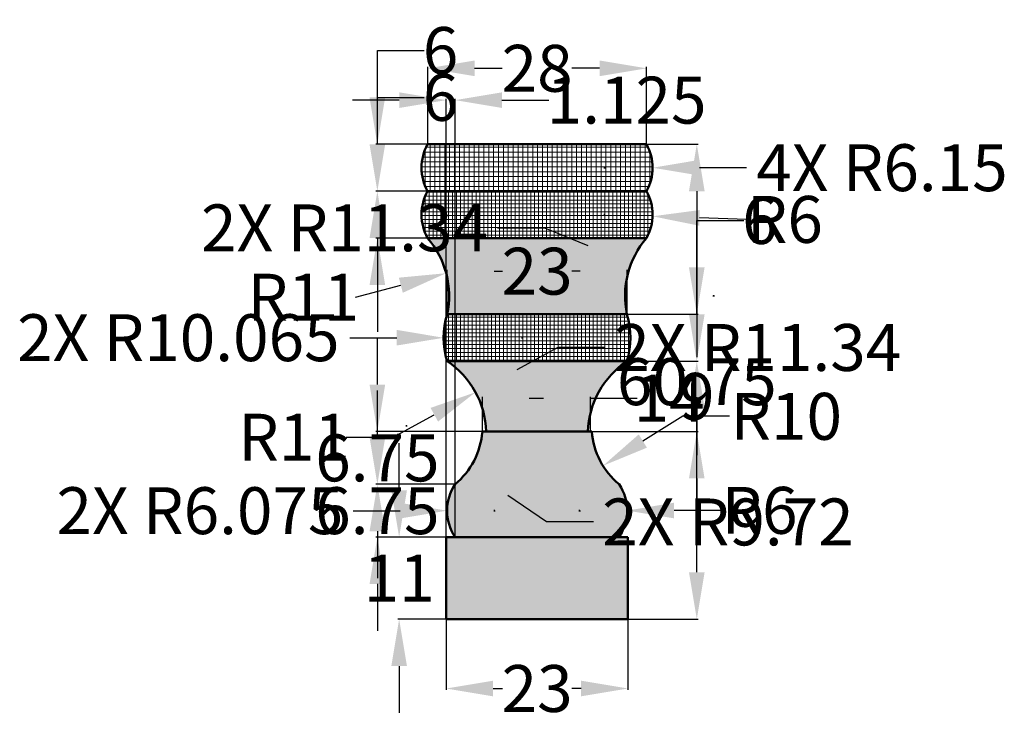
# Model space of a CAD drawing. Units: millimetres. Extents: x 141 to 267, y 101 to 190.
import ezdxf

# ---------------------------------------------------------------- set-up
doc = ezdxf.new("R2010")
doc.units = ezdxf.units.MM
doc.header["$MEASUREMENT"] = 0
for name, color, linetype, lineweight in [('M-DIMS', 2, 'Continuous', 25), ('M-HATC', 8, 'Continuous', 18), ('M-OUTL', 7, 'Continuous', 50)]:
    doc.layers.add(name, color=color, linetype=linetype, lineweight=lineweight)
doc.styles.get("Standard").update_dxf_attribs({"font": 'arial.ttf'})
doc.dimstyles.get("Standard").update_dxf_attribs({"dimtxt": 6, "dimasz": 6, "dimexe": 0.18, "dimexo": 0.0625, "dimgap": 0.09, "dimtad": 0, "dimtih": 1, "dimtoh": 1, "dimdec": 0, "dimzin": 0, "dimdsep": 46, "dimtxsty": 'Standard', "dimcen": 0.09, "dimadec": 0, "dimazin": 0, "dimtfac": 1, "dimtdec": 0, "dimtofl": 0, "dimtmove": 0, "dimatfit": 3, "dimfxl": 1, "dimtolj": 1, "dimtzin": 0, "dimarcsym": 0})

# ---------------------------------------------------------------- blocks, each defined once
blk = doc.blocks.new('*D1')
at = {"layer": 'Defpoints', "color": 0, "transparency": 16777216}
for p in [(195.71, 157.64), (184.75, 154.74)]:
    blk.add_point(p, dxfattribs=at)
at = {"layer": 'M-DIMS', "color": 0, "lineweight": -2, "transparency": 16777216}
blk.add_line((184.11, 154.57), (189.91, 156.11), dxfattribs=at)
at = {"layer": 'M-DIMS', "color": 0, "transparency": 16777216}
blk.add_solid([(189.66, 157.07), (190.17, 155.14), (195.71, 157.64)], dxfattribs=at)
at = {"layer": 'M-DIMS', "color": 0, "transparency": 16777216, "insert": (177.43, 154.57), "char_height": 6, "attachment_point": 5}
blk.add_mtext('\\A1;R11', dxfattribs=at)
blk = doc.blocks.new('*D2')
at = {"layer": 'Defpoints', "color": 0, "transparency": 16777216}
for p in [(199.47, 142.41), (189.51, 136.98)]:
    blk.add_point(p, dxfattribs=at)
at = {"layer": 'M-DIMS', "color": 0, "lineweight": -2, "transparency": 16777216}
for p, q in [((188.93, 136.66), (194.2, 139.54)), ((182.93, 136.66), (188.93, 136.66))]:
    blk.add_line(p, q, dxfattribs=at)
at = {"layer": 'M-DIMS', "color": 0, "transparency": 16777216}
blk.add_solid([(193.72, 140.41), (194.68, 138.66), (199.47, 142.41)], dxfattribs=at)
at = {"layer": 'M-DIMS', "color": 0, "transparency": 16777216, "insert": (176.25, 136.66), "char_height": 6, "attachment_point": 5}
blk.add_mtext('\\A1;R11', dxfattribs=at)
blk = doc.blocks.new('*D3')
at = {"layer": 'Defpoints', "color": 0, "transparency": 16777216}
for p in [(224.04, 138.13), (215.78, 133.01)]:
    blk.add_point(p, dxfattribs=at)
at = {"layer": 'M-DIMS', "color": 0, "lineweight": -2, "transparency": 16777216}
for p, q in [((225.98, 139.33), (220.88, 136.17)), ((231.98, 139.33), (225.98, 139.33))]:
    blk.add_line(p, q, dxfattribs=at)
at = {"layer": 'M-DIMS', "color": 0, "transparency": 16777216}
blk.add_solid([(220.35, 137.02), (221.4, 135.32), (215.78, 133.01)], dxfattribs=at)
at = {"layer": 'M-DIMS', "color": 0, "transparency": 16777216, "insert": (239.22, 139.33), "char_height": 6, "attachment_point": 5}
blk.add_mtext('\\A1;R10', dxfattribs=at)
blk = doc.blocks.new('*D4')
at = {"layer": 'Defpoints', "color": 0, "transparency": 16777216}
for p in [(212.79, 127.26), (218.87, 127.27)]:
    blk.add_point(p, dxfattribs=at)
at = {"layer": 'M-DIMS', "color": 0, "lineweight": -2, "transparency": 16777216}
for p, q in [((212.7, 127.26), (212.88, 127.26)), ((212.79, 127.17), (212.79, 127.35)), ((230.87, 127.3), (224.87, 127.28))]:
    blk.add_line(p, q, dxfattribs=at)
at = {"layer": 'M-DIMS', "color": 0, "transparency": 16777216}
blk.add_solid([(224.87, 128.28), (224.87, 126.28), (218.87, 127.27)], dxfattribs=at)
at = {"layer": 'M-DIMS', "color": 0, "transparency": 16777216, "insert": (235.8, 127.3), "char_height": 6, "attachment_point": 5}
blk.add_mtext('\\A1;R6', dxfattribs=at)
blk = doc.blocks.new('*D5')
at = {"layer": 'Defpoints', "color": 0, "transparency": 16777216}
for p in [(215.98, 165.13), (222.12, 164.92)]:
    blk.add_point(p, dxfattribs=at)
at = {"layer": 'M-DIMS', "color": 0, "lineweight": -2, "transparency": 16777216}
for p, q in [((215.89, 165.13), (216.07, 165.13)), ((215.98, 165.04), (215.98, 165.22)), ((234.12, 164.52), (228.12, 164.72))]:
    blk.add_line(p, q, dxfattribs=at)
at = {"layer": 'M-DIMS', "color": 0, "transparency": 16777216}
blk.add_solid([(228.15, 165.72), (228.09, 163.72), (222.12, 164.92)], dxfattribs=at)
at = {"layer": 'M-DIMS', "color": 0, "transparency": 16777216, "insert": (239.04, 164.52), "char_height": 6, "attachment_point": 5}
blk.add_mtext('\\A1;R6', dxfattribs=at)
blk = doc.blocks.new('*D6')
at = {"layer": 'Defpoints', "color": 0, "transparency": 16777216}
for p in [(195.72, 113.38), (218.97, 113.38), (218.97, 104.51)]:
    blk.add_point(p, dxfattribs=at)
at = {"layer": 'M-DIMS', "color": 0, "lineweight": -2, "transparency": 16777216}
for p, q in [((195.72, 113.32), (195.72, 104.33)), ((218.97, 113.32), (218.97, 104.33)), ((201.72, 104.51), (202.91, 104.51)), ((212.97, 104.51), (211.78, 104.51))]:
    blk.add_line(p, q, dxfattribs=at)
at = {"layer": 'M-DIMS', "color": 0, "transparency": 16777216}
for points in [[(201.72, 105.51), (201.72, 103.51), (195.72, 104.51)], [(212.97, 105.51), (212.97, 103.51), (218.97, 104.51)]]:
    blk.add_solid(points, dxfattribs=at)
at = {"layer": 'M-DIMS', "color": 0, "transparency": 16777216, "insert": (207.35, 104.51), "char_height": 6, "attachment_point": 5}
blk.add_mtext('\\A1;23', dxfattribs=at)
blk = doc.blocks.new('*D7')
at = {"layer": 'Defpoints', "color": 0, "transparency": 16777216}
for p in [(218.97, 123.88), (189.7, 113.38), (218.97, 113.38)]:
    blk.add_point(p, dxfattribs=at)
at = {"layer": 'M-DIMS', "color": 0, "lineweight": -2, "transparency": 16777216}
for p, q in [((189.7, 129.88), (189.7, 135.88)), ((218.91, 123.88), (189.52, 123.88)), ((218.91, 113.38), (189.52, 113.38)), ((189.7, 107.38), (189.7, 101.38))]:
    blk.add_line(p, q, dxfattribs=at)
at = {"layer": 'M-DIMS', "color": 0, "transparency": 16777216}
for points in [[(188.7, 129.88), (190.7, 129.88), (189.7, 123.88)], [(188.7, 107.38), (190.7, 107.38), (189.7, 113.38)]]:
    blk.add_solid(points, dxfattribs=at)
at = {"layer": 'M-DIMS', "color": 0, "transparency": 16777216, "insert": (189.7, 118.63), "char_height": 6, "attachment_point": 5}
blk.add_mtext('\\A1;11', dxfattribs=at)
blk = doc.blocks.new('*D8')
at = {"layer": 'Defpoints', "color": 0, "transparency": 16777216}
for p in [(221.35, 183.85), (193.35, 174.13), (221.35, 174.13)]:
    blk.add_point(p, dxfattribs=at)
at = {"layer": 'M-DIMS', "color": 0, "lineweight": -2, "transparency": 16777216}
for p, q in [((193.35, 174.2), (193.35, 184.03)), ((221.35, 174.2), (221.35, 184.03)), ((199.35, 183.85), (202.9, 183.85)), ((215.35, 183.85), (211.79, 183.85))]:
    blk.add_line(p, q, dxfattribs=at)
at = {"layer": 'M-DIMS', "color": 0, "transparency": 16777216}
for points in [[(199.35, 184.85), (199.35, 182.85), (193.35, 183.85)], [(215.35, 184.85), (215.35, 182.85), (221.35, 183.85)]]:
    blk.add_solid(points, dxfattribs=at)
at = {"layer": 'M-DIMS', "color": 0, "transparency": 16777216, "insert": (207.35, 183.85), "char_height": 6, "attachment_point": 5}
blk.add_mtext('\\A1;28', dxfattribs=at)
blk = doc.blocks.new('*D9')
at = {"layer": 'Defpoints', "color": 0, "transparency": 16777216}
for p in [(214.16, 141.66), (200.35, 137.38), (214.16, 137.38)]:
    blk.add_point(p, dxfattribs=at)
at = {"layer": 'M-DIMS', "color": 0, "lineweight": -2, "transparency": 16777216}
for p, q in [((200.35, 137.45), (200.35, 141.84)), ((206.35, 141.66), (208.16, 141.66)), ((214.16, 137.45), (214.16, 141.84)), ((214.16, 141.66), (220.16, 141.66))]:
    blk.add_line(p, q, dxfattribs=at)
at = {"layer": 'M-DIMS', "color": 0, "transparency": 16777216}
for points in [[(206.35, 142.66), (206.35, 140.66), (200.35, 141.66)], [(208.16, 142.66), (208.16, 140.66), (214.16, 141.66)]]:
    blk.add_solid(points, dxfattribs=at)
at = {"layer": 'M-DIMS', "color": 0, "transparency": 16777216, "insert": (224.25, 141.66), "char_height": 6, "attachment_point": 5}
blk.add_mtext('\\A1;14', dxfattribs=at)
blk = doc.blocks.new('*D10')
at = {"layer": 'Defpoints', "color": 0, "transparency": 16777216}
for p in [(218.85, 157.9), (195.85, 152.38), (218.85, 152.38)]:
    blk.add_point(p, dxfattribs=at)
at = {"layer": 'M-DIMS', "color": 0, "lineweight": -2, "transparency": 16777216}
for p, q in [((195.85, 152.45), (195.85, 158.08)), ((201.85, 157.9), (202.91, 157.9)), ((212.85, 157.9), (211.78, 157.9)), ((218.85, 152.45), (218.85, 158.08))]:
    blk.add_line(p, q, dxfattribs=at)
at = {"layer": 'M-DIMS', "color": 0, "transparency": 16777216}
for points in [[(201.85, 158.9), (201.85, 156.9), (195.85, 157.9)], [(212.85, 158.9), (212.85, 156.9), (218.85, 157.9)]]:
    blk.add_solid(points, dxfattribs=at)
at = {"layer": 'M-DIMS', "color": 0, "transparency": 16777216, "insert": (207.35, 157.9), "char_height": 6, "attachment_point": 5}
blk.add_mtext('\\A1;23', dxfattribs=at)
blk = doc.blocks.new('*D11')
at = {"layer": 'Defpoints', "color": 0, "transparency": 16777216}
for p in [(221.35, 174.13), (227.78, 174.13), (218.97, 113.38)]:
    blk.add_point(p, dxfattribs=at)
at = {"layer": 'M-DIMS', "color": 0, "lineweight": -2, "transparency": 16777216}
for p, q in [((221.41, 174.13), (227.96, 174.13)), ((227.78, 168.13), (227.78, 146.91)), ((227.78, 119.38), (227.78, 140.61)), ((219.03, 113.38), (227.96, 113.38))]:
    blk.add_line(p, q, dxfattribs=at)
at = {"layer": 'M-DIMS', "color": 0, "transparency": 16777216}
for points in [[(226.78, 168.13), (228.78, 168.13), (227.78, 174.13)], [(226.78, 119.38), (228.78, 119.38), (227.78, 113.38)]]:
    blk.add_solid(points, dxfattribs=at)
at = {"layer": 'M-DIMS', "color": 0, "transparency": 16777216, "insert": (227.78, 143.76), "char_height": 6, "attachment_point": 5}
blk.add_mtext('\\A1;60.75', dxfattribs=at)
blk = doc.blocks.new('*D12')
at = {"layer": 'Defpoints', "color": 0, "transparency": 16777216}
for p in [(186.914449, 130.634532), (196.84579, 130.634532), (196.84579, 123.884532)]:
    blk.add_point(p, dxfattribs=at)
at = {"layer": 'M-DIMS', "color": 0, "lineweight": -2, "transparency": 16777216}
for p, q in [((186.914449, 136.634532), (186.914449, 142.634532)), ((196.78329, 130.634532), (186.734449, 130.634532)), ((196.78329, 123.884532), (186.734449, 123.884532)), ((186.914449, 117.884532), (186.914449, 111.884532))]:
    blk.add_line(p, q, dxfattribs=at)
at = {"layer": 'M-DIMS', "color": 0, "transparency": 16777216}
for points in [[(185.914449, 136.634532), (187.914449, 136.634532), (186.914449, 130.634532)], [(185.914449, 117.884532), (187.914449, 117.884532), (186.914449, 123.884532)]]:
    blk.add_solid(points, dxfattribs=at)
at = {"layer": 'M-DIMS', "color": 0, "transparency": 16777216, "insert": (186.914449, 127.259532), "char_height": 6, "attachment_point": 5}
blk.add_mtext('\\A1;6.75', dxfattribs=at)
blk = doc.blocks.new('*D13')
at = {"layer": 'Defpoints', "color": 0, "transparency": 16777216}
for p in [(186.914449, 137.384532), (200.34579, 137.384532), (196.84579, 130.634532)]:
    blk.add_point(p, dxfattribs=at)
at = {"layer": 'M-DIMS', "color": 0, "lineweight": -2, "transparency": 16777216}
for p, q in [((186.914449, 143.384532), (186.914449, 149.384532)), ((200.28329, 137.384532), (186.734449, 137.384532)), ((196.78329, 130.634532), (186.734449, 130.634532)), ((186.914449, 124.634532), (186.914449, 118.634532))]:
    blk.add_line(p, q, dxfattribs=at)
at = {"layer": 'M-DIMS', "color": 0, "transparency": 16777216}
for points in [[(185.914449, 143.384532), (187.914449, 143.384532), (186.914449, 137.384532)], [(185.914449, 124.634532), (187.914449, 124.634532), (186.914449, 130.634532)]]:
    blk.add_solid(points, dxfattribs=at)
at = {"layer": 'M-DIMS', "color": 0, "transparency": 16777216, "insert": (186.914449, 134.009532), "char_height": 6, "attachment_point": 5}
blk.add_mtext('\\A1;6.75', dxfattribs=at)
blk = doc.blocks.new('*D14')
at = {"layer": 'Defpoints', "color": 0, "transparency": 16777216}
for p in [(218.84579, 146.384532), (227.777131, 146.384532), (214.34579, 137.384532)]:
    blk.add_point(p, dxfattribs=at)
at = {"layer": 'M-DIMS', "color": 0, "lineweight": -2, "transparency": 16777216}
for p, q in [((227.777131, 152.384532), (227.777131, 158.384532)), ((218.90829, 146.384532), (227.957131, 146.384532)), ((214.40829, 137.384532), (227.957131, 137.384532)), ((227.777131, 131.384532), (227.777131, 125.384532))]:
    blk.add_line(p, q, dxfattribs=at)
at = {"layer": 'M-DIMS', "color": 0, "transparency": 16777216}
for points in [[(226.777131, 152.384532), (228.777131, 152.384532), (227.777131, 146.384532)], [(226.777131, 131.384532), (228.777131, 131.384532), (227.777131, 137.384532)]]:
    blk.add_solid(points, dxfattribs=at)
at = {"layer": 'M-DIMS', "color": 0, "transparency": 16777216, "insert": (227.777131, 141.884532), "char_height": 6, "attachment_point": 5}
blk.add_mtext('\\A1;9', dxfattribs=at)
blk = doc.blocks.new('*D15')
at = {"layer": 'Defpoints', "color": 0, "transparency": 16777216}
for p in [(196.85, 179.78), (195.72, 123.88), (196.85, 123.88)]:
    blk.add_point(p, dxfattribs=at)
at = {"layer": 'M-DIMS', "color": 0, "lineweight": -2, "transparency": 16777216}
for p, q in [((189.72, 179.78), (183.72, 179.78)), ((195.72, 123.95), (195.72, 179.96)), ((196.85, 123.95), (196.85, 179.96)), ((202.85, 179.78), (208.85, 179.78))]:
    blk.add_line(p, q, dxfattribs=at)
at = {"layer": 'M-DIMS', "color": 0, "transparency": 16777216}
for points in [[(189.72, 180.78), (189.72, 178.78), (195.72, 179.78)], [(202.85, 180.78), (202.85, 178.78), (196.85, 179.78)]]:
    blk.add_solid(points, dxfattribs=at)
at = {"layer": 'M-DIMS', "color": 0, "transparency": 16777216, "insert": (218.8, 179.78), "char_height": 6, "attachment_point": 5}
blk.add_mtext('\\A1;1.125', dxfattribs=at)
blk = doc.blocks.new('*D16')
at = {"layer": 'Defpoints', "color": 0, "transparency": 16777216}
for p in [(218.85, 152.38), (227.78, 152.38), (218.85, 146.38)]:
    blk.add_point(p, dxfattribs=at)
at = {"layer": 'M-DIMS', "color": 0, "lineweight": -2, "transparency": 16777216}
for p, q in [((227.78, 158.38), (227.78, 164.38)), ((227.78, 164.38), (233.78, 164.38)), ((218.91, 152.38), (227.96, 152.38)), ((218.91, 146.38), (227.96, 146.38)), ((227.78, 140.38), (227.78, 134.38))]:
    blk.add_line(p, q, dxfattribs=at)
at = {"layer": 'M-DIMS', "color": 0, "transparency": 16777216}
for points in [[(226.78, 158.38), (228.78, 158.38), (227.78, 152.38)], [(226.78, 140.38), (228.78, 140.38), (227.78, 146.38)]]:
    blk.add_solid(points, dxfattribs=at)
at = {"layer": 'M-DIMS', "color": 0, "transparency": 16777216, "insert": (235.85, 164.38), "char_height": 6, "attachment_point": 5}
blk.add_mtext('\\A1;6', dxfattribs=at)
blk = doc.blocks.new('*D17')
at = {"layer": 'Defpoints', "color": 0, "transparency": 16777216}
for p in [(186.91, 168.13), (193.35, 168.13), (193.35, 162.13)]:
    blk.add_point(p, dxfattribs=at)
at = {"layer": 'M-DIMS', "color": 0, "lineweight": -2, "transparency": 16777216}
for p, q in [((186.91, 174.13), (186.91, 180.13)), ((186.91, 180.13), (192.91, 180.13)), ((193.28, 168.13), (186.73, 168.13)), ((193.28, 162.13), (186.73, 162.13)), ((186.91, 156.13), (186.91, 150.13))]:
    blk.add_line(p, q, dxfattribs=at)
at = {"layer": 'M-DIMS', "color": 0, "transparency": 16777216}
for points in [[(185.91, 174.13), (187.91, 174.13), (186.91, 168.13)], [(185.91, 156.13), (187.91, 156.13), (186.91, 162.13)]]:
    blk.add_solid(points, dxfattribs=at)
at = {"layer": 'M-DIMS', "color": 0, "transparency": 16777216, "insert": (194.99, 180.13), "char_height": 6, "attachment_point": 5}
blk.add_mtext('\\A1;6', dxfattribs=at)
blk = doc.blocks.new('*D18')
at = {"layer": 'Defpoints', "color": 0, "transparency": 16777216}
for p in [(186.91, 174.13), (193.35, 174.13), (193.35, 168.13)]:
    blk.add_point(p, dxfattribs=at)
at = {"layer": 'M-DIMS', "color": 0, "lineweight": -2, "transparency": 16777216}
for p, q in [((186.91, 180.13), (186.91, 186.13)), ((186.91, 186.13), (192.91, 186.13)), ((193.28, 174.13), (186.73, 174.13)), ((193.28, 168.13), (186.73, 168.13)), ((186.91, 162.13), (186.91, 156.13))]:
    blk.add_line(p, q, dxfattribs=at)
at = {"layer": 'M-DIMS', "color": 0, "transparency": 16777216}
for points in [[(185.91, 180.13), (187.91, 180.13), (186.91, 174.13)], [(185.91, 162.13), (187.91, 162.13), (186.91, 168.13)]]:
    blk.add_solid(points, dxfattribs=at)
at = {"layer": 'M-DIMS', "color": 0, "transparency": 16777216, "insert": (194.99, 186.13), "char_height": 6, "attachment_point": 5}
blk.add_mtext('\\A1;6', dxfattribs=at)
blk = doc.blocks.new('*D19')
at = {"layer": 'Defpoints', "color": 0, "transparency": 16777216}
for p in [(195.39, 149.38), (205.45, 149.38)]:
    blk.add_point(p, dxfattribs=at)
at = {"layer": 'M-DIMS', "color": 0, "lineweight": -2, "transparency": 16777216}
for p, q in [((183.39, 149.39), (189.39, 149.39)), ((205.36, 149.38), (205.54, 149.38)), ((205.45, 149.29), (205.45, 149.47))]:
    blk.add_line(p, q, dxfattribs=at)
at = {"layer": 'M-DIMS', "color": 0, "transparency": 16777216}
blk.add_solid([(189.39, 150.39), (189.39, 148.39), (195.39, 149.38)], dxfattribs=at)
at = {"layer": 'M-DIMS', "color": 0, "transparency": 16777216, "insert": (161.45, 149.39), "char_height": 6, "attachment_point": 5}
blk.add_mtext('\\A1;2X R10.065', dxfattribs=at)
blk = doc.blocks.new('*D20')
at = {"layer": 'Defpoints', "color": 0, "transparency": 16777216}
for p in [(215.98, 171.13), (222.13, 171.13)]:
    blk.add_point(p, dxfattribs=at)
at = {"layer": 'M-DIMS', "color": 0, "lineweight": -2, "transparency": 16777216}
for p, q in [((215.89, 171.13), (216.07, 171.13)), ((215.98, 171.04), (215.98, 171.22)), ((234.13, 171.14), (228.13, 171.14))]:
    blk.add_line(p, q, dxfattribs=at)
at = {"layer": 'M-DIMS', "color": 0, "transparency": 16777216}
blk.add_solid([(228.13, 172.14), (228.13, 170.14), (222.13, 171.13)], dxfattribs=at)
at = {"layer": 'M-DIMS', "color": 0, "transparency": 16777216, "insert": (251.47, 171.14), "char_height": 6, "attachment_point": 5}
blk.add_mtext('\\A1;4X R6.15', dxfattribs=at)
blk = doc.blocks.new('*D21')
at = {"layer": 'Defpoints', "color": 0, "transparency": 16777216}
for p in [(195.82, 127.26), (201.9, 127.26)]:
    blk.add_point(p, dxfattribs=at)
at = {"layer": 'M-DIMS', "color": 0, "lineweight": -2, "transparency": 16777216}
for p, q in [((183.82, 127.26), (189.82, 127.26)), ((201.81, 127.26), (201.99, 127.26)), ((201.9, 127.17), (201.9, 127.35))]:
    blk.add_line(p, q, dxfattribs=at)
at = {"layer": 'M-DIMS', "color": 0, "transparency": 16777216}
blk.add_solid([(189.82, 128.26), (189.82, 126.26), (195.82, 127.26)], dxfattribs=at)
at = {"layer": 'M-DIMS', "color": 0, "transparency": 16777216, "insert": (164.22, 127.26), "char_height": 6, "attachment_point": 5}
blk.add_mtext('\\A1;2X R6.075', dxfattribs=at)
blk = doc.blocks.new('*D22')
at = {"layer": 'Defpoints', "color": 0, "transparency": 16777216}
for p in [(219.42, 158.96), (229.94, 154.74)]:
    blk.add_point(p, dxfattribs=at)
at = {"layer": 'M-DIMS', "color": 0, "lineweight": -2, "transparency": 16777216}
for p, q in [((202.28, 163.44), (208.28, 163.44)), ((208.28, 163.44), (213.85, 161.2)), ((229.85, 154.74), (230.03, 154.74)), ((229.94, 154.65), (229.94, 154.83))]:
    blk.add_line(p, q, dxfattribs=at)
at = {"layer": 'M-DIMS', "color": 0, "transparency": 16777216}
blk.add_solid([(214.22, 162.13), (213.48, 160.27), (219.42, 158.96)], dxfattribs=at)
at = {"layer": 'M-DIMS', "color": 0, "transparency": 16777216, "insert": (182.71, 163.44), "char_height": 6, "attachment_point": 5}
blk.add_mtext('\\A1;2X R11.34', dxfattribs=at)
blk = doc.blocks.new('*D23')
at = {"layer": 'Defpoints', "color": 0, "transparency": 16777216}
for p in [(199.47, 142.4), (189.51, 136.98)]:
    blk.add_point(p, dxfattribs=at)
at = {"layer": 'M-DIMS', "color": 0, "lineweight": -2, "transparency": 16777216}
for p, q in [((210.01, 148.14), (204.74, 145.27)), ((216.01, 148.14), (210.01, 148.14)), ((189.42, 136.98), (189.6, 136.98)), ((189.51, 136.89), (189.51, 137.07))]:
    blk.add_line(p, q, dxfattribs=at)
at = {"layer": 'M-DIMS', "color": 0, "transparency": 16777216}
blk.add_solid([(204.26, 146.15), (205.22, 144.39), (199.47, 142.4)], dxfattribs=at)
at = {"layer": 'M-DIMS', "color": 0, "transparency": 16777216, "insert": (235.58, 148.14), "char_height": 6, "attachment_point": 5}
blk.add_mtext('\\A1;2X R11.34', dxfattribs=at)
blk = doc.blocks.new('*D24')
at = {"layer": 'Defpoints', "color": 0, "transparency": 16777216}
for p in [(190.65, 138.13), (198.66, 132.62)]:
    blk.add_point(p, dxfattribs=at)
at = {"layer": 'M-DIMS', "color": 0, "lineweight": -2, "transparency": 16777216}
for p, q in [((190.56, 138.13), (190.74, 138.13)), ((190.65, 138.04), (190.65, 138.22)), ((208.55, 125.82), (203.61, 129.22)), ((214.55, 125.82), (208.55, 125.82))]:
    blk.add_line(p, q, dxfattribs=at)
at = {"layer": 'M-DIMS', "color": 0, "transparency": 16777216}
blk.add_solid([(204.17, 130.04), (203.04, 128.39), (198.66, 132.62)], dxfattribs=at)
at = {"layer": 'M-DIMS', "color": 0, "transparency": 16777216, "insert": (231.77, 125.82), "char_height": 6, "attachment_point": 5}
blk.add_mtext('\\A1;2X R9.72', dxfattribs=at)

msp = doc.modelspace()

# ---------------------------------------------------------------- hatches: boundary and pattern name
at = {"layer": 'M-HATC'}
h = msp.add_hatch(dxfattribs=at)
h.set_pattern_fill('NET', color=256, scale=5)
h.set_pattern_definition([(0, (183.0333, 110.00186), (0, 0.625), []), (90, (183.0333, 110.00186), (-0.625, 0), [])])
h.paths.add_polyline_path([(193.3458, 174.1345, 0.26044698), (193.3458, 168.1345), (207.3458, 168.1345), (221.3458, 168.1345, 0.26044698), (221.3458, 174.1345), (207.3458, 174.1345)])
h = msp.add_hatch(dxfattribs=at)
h.set_pattern_fill('NET', color=256, scale=4)
h.set_pattern_definition([(0, (183.0333, 110.00186), (0, 0.5), []), (90, (183.0333, 110.00186), (-0.5, 0), [])])
h.paths.add_polyline_path([(221.3458, 162.1345, 0.26044698), (221.3458, 168.1345), (207.3458, 168.1345), (193.3458, 168.1345, 0.26044698), (193.3458, 162.1345), (207.3458, 162.1345)])
h.paths.add_polyline_path([(207.3458, 146.3845), (214.3458, 146.3845), (218.8458, 146.3845, 0.15249707), (218.8458, 152.3845), (207.3458, 152.3845), (195.8458, 152.3845, 0.15249707), (195.8458, 146.3845)])
h = msp.add_hatch(color=256, dxfattribs=at)
h.dxf.hatch_style = 1
h.set_gradient(color1=(188, 108, 11), name='CYLINDER')
h.paths.add_polyline_path([(207.3458, 162.1345), (193.3458, 162.1345, -0.2340569), (195.8458, 152.3845), (207.3458, 152.3845), (218.8458, 152.3845, -0.2340569), (221.3458, 162.1345)])
h.paths.add_polyline_path([(213.8458, 137.3845, -0.24005588), (218.8458, 146.3845), (207.3458, 146.3845), (200.3458, 146.3845), (195.8458, 146.3845, -0.24005588), (200.8458, 137.3845)])
h = msp.add_hatch(color=256, dxfattribs=at)
h.dxf.hatch_style = 1
h.set_gradient(color1=(188, 108, 11), name='CYLINDER')
h.paths.add_polyline_path([(217.8458, 123.8845, 0.30333705), (217.8458, 130.6345, -0.20367464), (214.3458, 137.3845), (200.3458, 137.3845, -0.20367464), (196.8458, 130.6345, 0.30333705), (196.8458, 123.8845)])
h.paths.add_polyline_path([(218.9708, 113.3845), (218.9708, 123.8845), (195.7208, 123.8845), (195.7208, 113.3845)])

# ---------------------------------------------------------------- linework, layer by layer
at = {"layer": 'M-OUTL'}
for p, q in [((207.3458, 174.1345), (193.3458, 174.1345)), ((207.3458, 174.1345), (221.3458, 174.1345)), ((207.3458, 168.1345), (193.3458, 168.1345)), ((207.3458, 168.1345), (193.3458, 168.1345)), ((207.3458, 168.1345), (221.3458, 168.1345)), ((207.3458, 168.1345), (221.3458, 168.1345)), ((207.3458, 162.1345), (193.3458, 162.1345)), ((207.3458, 162.1345), (195.8458, 162.1345)), ((207.3458, 162.1345), (218.8458, 162.1345)), ((207.3458, 162.1345), (221.3458, 162.1345)), ((207.3458, 152.3845), (195.8458, 152.3845)), ((207.3458, 152.3845), (218.8458, 152.3845)), ((207.3458, 146.3845), (195.8458, 146.3845)), ((200.3458, 146.3845), (214.3458, 146.3845)), ((207.3458, 146.3845), (218.8458, 146.3845)), ((207.3458, 137.3845), (200.3458, 137.3845)), ((200.3458, 137.3845), (214.3458, 137.3845)), ((207.3458, 137.3845), (200.8458, 137.3845)), ((207.3458, 137.3845), (214.3458, 137.3845)), ((207.3458, 137.3845), (213.8458, 137.3845)), ((195.7208, 123.8845), (218.9708, 123.8845)), ((195.7208, 123.8845), (195.7208, 113.3845)), ((218.9708, 123.8845), (218.9708, 113.3845)), ((195.7208, 113.3845), (218.9708, 113.3845))]:
    msp.add_line(p, q, dxfattribs=at)
for centre, radius, start, end in [((198.7144, 171.1345), 6.15, 150.803596, 209.196404), ((215.9771, 171.1345), 6.15, 330.803596, 29.196404), ((198.7144, 165.1345), 6.15, 150.803596, 209.196404), ((215.9771, 165.1345), 6.15, 330.803596, 29.196404), ((184.7522, 154.7355), 11.34, 348.03473, 40.72806), ((229.9394, 154.7355), 11.34, 139.27194, 191.96527), ((205.4533, 149.3845), 10.065, 162.658725, 197.341275), ((209.2383, 149.3845), 10.065, 342.658725, 17.341275), ((189.5131, 136.9775), 11.34, 2.057083, 56.052125), ((225.1785, 136.9775), 11.34, 123.947875, 177.942917), ((190.6542, 138.1274), 9.72, 309.56796, 355.616889), ((224.0374, 138.1274), 9.72, 184.383111, 230.43204), ((201.897, 127.2595), 6.075, 146.251011, 213.748989), ((212.7946, 127.2595), 6.075, 326.251011, 33.748989)]:
    msp.add_arc(centre, radius, start, end, dxfattribs=at)

# ---------------------------------------------------------------- dimensions: what is measured, and where the dimension line sits
at = {"layer": 'M-DIMS'}
for base, p1, p2, override, picture, middle in [((186.9144, 174.1345), (193.3458, 168.1345), (193.3458, 174.1345), {"dimdec": 0, "dimlfac": 1, "dimrnd": 0, "dimzin": 0, "dimdsep": 46, "dimlunit": 2}, '*D18', (194.9853, 186.1345)), ((186.9144, 168.1345), (193.3458, 162.1345), (193.3458, 168.1345), {"dimdec": 0, "dimlfac": 1, "dimrnd": 0, "dimzin": 0, "dimdsep": 46, "dimlunit": 2}, '*D17', (194.9853, 180.1345)), ((227.7771, 174.1345), (218.9708, 113.3845), (221.3458, 174.1345), {"dimdec": 2, "dimlfac": 1, "dimrnd": 0, "dimzin": 0, "dimdsep": 46, "dimlunit": 2}, '*D11', (227.7771, 143.7595)), ((227.7771, 152.3845), (218.8458, 146.3845), (218.8458, 152.3845), {"dimdec": 0, "dimlfac": 1, "dimrnd": 0, "dimzin": 0, "dimdsep": 46, "dimlunit": 2}, '*D16', (235.848, 164.3845)), ((227.7771, 146.3845), (214.3458, 137.3845), (218.8458, 146.3845), {"dimdec": 0, "dimlfac": 1, "dimrnd": 0, "dimzin": 0, "dimdsep": 46, "dimlunit": 2}, '*D14', (227.7771, 141.8845)), ((186.9144, 137.3845), (196.8458, 130.6345), (200.3458, 137.3845), {"dimdec": 2, "dimlfac": 1, "dimrnd": 0, "dimzin": 0, "dimdsep": 46, "dimlunit": 2}, '*D13', (186.9144, 134.0095)), ((186.9144, 130.6345), (196.8458, 123.8845), (196.8458, 130.6345), {"dimdec": 2, "dimlfac": 1, "dimrnd": 0, "dimzin": 0, "dimdsep": 46, "dimlunit": 2}, '*D12', (186.9144, 127.2595)), ((189.6964867617, 113.3845320239), (218.9707902531, 123.8845320239), (218.9707902531, 113.3845320239), {"dimclrd": 0, "dimclre": 0, "dimclrt": 0}, '*D7', (189.6964867617, 118.6345320239))]:
    dim = msp.add_linear_dim(base=base, p1=p1, p2=p2, angle=90, dimstyle='Standard', override=override, dxfattribs=at)
    dim.commit()
    dim.dimension.update_dxf_attribs({"geometry": picture, "text_midpoint": middle})
for base, p1, p2, override, picture, middle in [((221.3458, 183.8482), (193.3458, 174.1345), (221.3458, 174.1345), {"dimclrd": 0, "dimclre": 0, "dimclrt": 0}, '*D8', (207.3458, 183.8482)), ((196.8458, 179.7845), (195.7208, 123.8845), (196.8458, 123.8845), {"dimdec": 3, "dimlfac": 1, "dimrnd": 0, "dimzin": 0, "dimdsep": 46, "dimlunit": 2}, '*D15', (218.7994, 179.7845)), ((218.8458, 157.9018), (195.8458, 152.3845), (218.8458, 152.3845), {"dimclrd": 0, "dimclre": 0, "dimclrt": 0}, '*D10', (207.3458, 157.9018)), ((214.1577, 141.6608), (200.3458, 137.3845), (214.1577, 137.3845), {"dimclrd": 0, "dimclre": 0, "dimclrt": 0}, '*D9', (224.2504, 141.6608)), ((218.9708, 104.5082), (195.7208, 113.3845), (218.9708, 113.3845), {"dimclrd": 0, "dimclre": 0, "dimclrt": 0}, '*D6', (207.3458, 104.5082))]:
    dim = msp.add_linear_dim(base=base, p1=p1, p2=p2, dimstyle='Standard', override=override, dxfattribs=at)
    dim.commit()
    dim.dimension.update_dxf_attribs({"geometry": picture, "text_midpoint": middle})
for center, mpoint, text, override, picture, middle in [((215.9771, 171.1345), (222.1271, 171.135), '4X <>', {"dimdec": 2, "dimlfac": 1, "dimrnd": 0, "dimzin": 0, "dimdsep": 46, "dimlunit": 2}, '*D20', (251.4702, 171.1359)), ((229.9394, 154.7355), (219.417, 158.9633), '2X <>', {"dimdec": 2, "dimlfac": 1, "dimrnd": 0, "dimzin": 0, "dimdsep": 46, "dimlunit": 2}, '*D22', (182.7126, 163.4371)), ((205.4533, 149.3845), (195.3883, 149.385), '2X <>', {"dimdec": 3, "dimlfac": 1, "dimrnd": 0, "dimzin": 0, "dimdsep": 46, "dimlunit": 2}, '*D19', (161.4531, 149.3856)), ((189.5131, 136.9775), (199.4714, 142.4023), '2X <>', {"dimdec": 2, "dimlfac": 1, "dimrnd": 0, "dimzin": 0, "dimdsep": 46, "dimlunit": 2}, '*D23', (235.5787, 148.1428)), ((190.6542, 138.1274), (198.6626, 132.6188), '2X <>', {"dimdec": 2, "dimlfac": 1, "dimrnd": 0, "dimzin": 0, "dimdsep": 46, "dimlunit": 2}, '*D24', (231.7698, 125.8182)), ((201.897, 127.2595), (195.822, 127.26), '2X <>', {"dimdec": 3, "dimlfac": 1, "dimrnd": 0, "dimzin": 0, "dimdsep": 46, "dimlunit": 2}, '*D21', (164.2177, 127.2609))]:
    dim = msp.add_radius_dim(center=center, mpoint=mpoint, text=text, dimstyle='Standard', override=override, dxfattribs=at)
    dim.commit()
    dim.dimension.update_dxf_attribs({"geometry": picture, "text_midpoint": middle})
for center, mpoint, picture, middle in [((215.9771, 165.1345), (222.1236, 164.9248), '*D5', (239.0422, 164.5155)), ((212.7946, 127.2595), (218.8695, 127.2718), '*D4', (235.7951, 127.2961))]:
    dim = msp.add_radius_dim(center=center, mpoint=mpoint, dimstyle='Standard', override={"dimclrd": 0, "dimclre": 0, "dimclrt": 0}, dxfattribs=at)
    dim.commit()
    dim.dimension.update_dxf_attribs({"geometry": picture, "text_midpoint": middle})
for center, mpoint, picture, middle in [((184.7522, 154.7355), (195.7127, 157.6445), '*D1', (184.1143, 154.5662)), ((189.5131, 136.9775), (199.4678, 142.4088), '*D2', (176.2544, 136.6614)), ((224.0374, 138.1274), (215.7757, 133.0064), '*D3', (239.2235, 139.3286))]:
    dim = msp.add_radius_dim(center=center, mpoint=mpoint, dimstyle='Standard', override={"dimclrd": 0, "dimclre": 0, "dimclrt": 0}, dxfattribs=at)
    dim.commit()
    dim.dimension.update_dxf_attribs({"geometry": picture, "text_midpoint": middle, "dimtype": 164})

doc.saveas('drawing.dxf')
